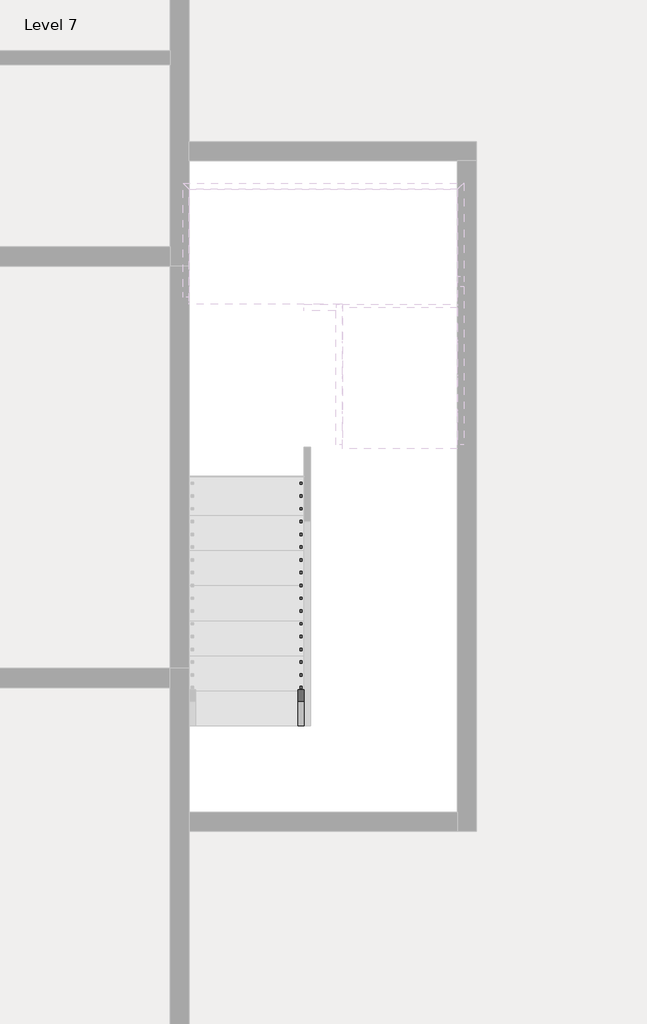
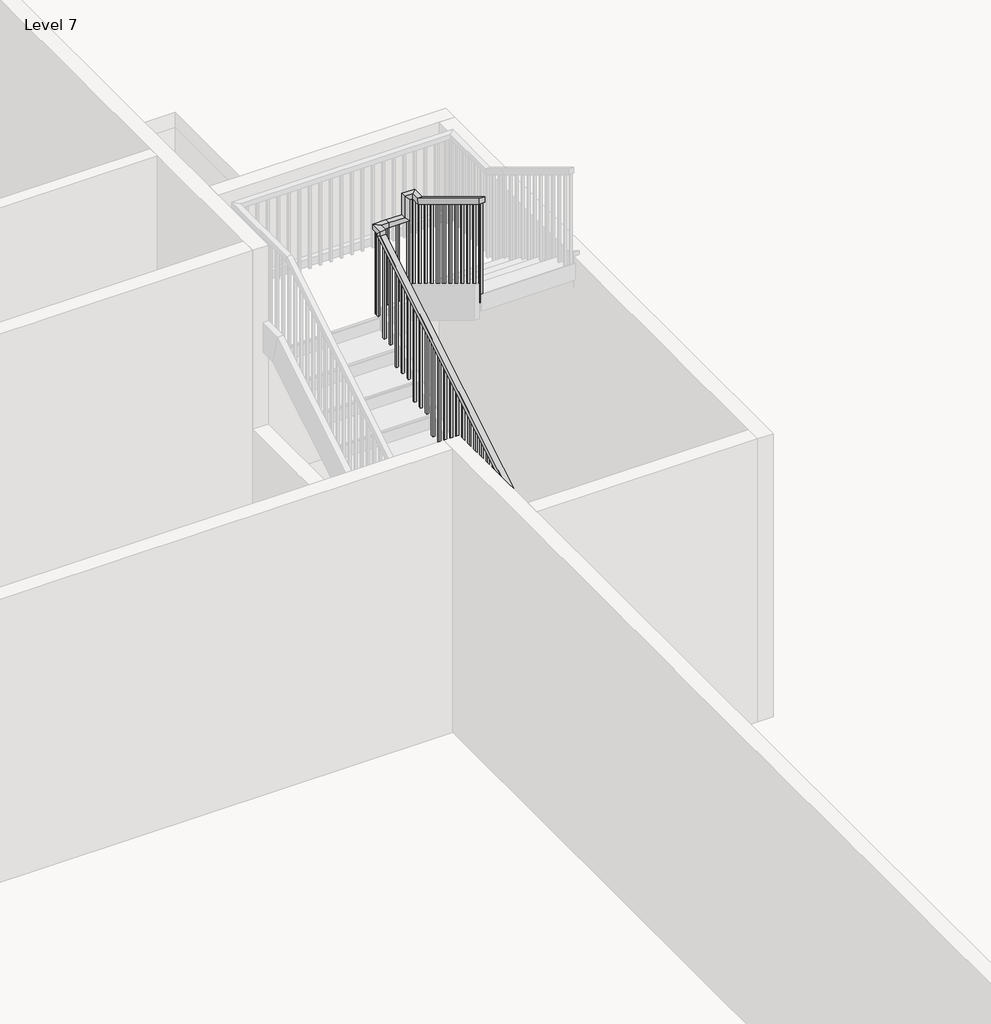
# One storey, part 7 of 8: 1 railing.
"""IFC4 building model written with IfcOpenShell, lengths in millimetres."""

from ifc_helpers import new_model, si_unit, frame, origin, place, context, project, spatial, polyline, outline, extrude, faceted_brep, element, save

model = new_model("IFC4")

# Units and contexts
model_context = context("Model", 3, world=origin())
ifc_project = project(units=[si_unit("LENGTHUNIT", "METRE", prefix="MILLI")], contexts=[model_context])

# Site, building, storey
site = spatial("IfcSite", under=ifc_project)
building = spatial("IfcBuilding", under=site)
storey = spatial("IfcBuildingStorey", under=building, Name="Level 7", Elevation=43522.6172466)

# Railing
placement = place(None, origin())
element("IfcRailing", 1, ObjectType="Handrail - Rectangular", at=placement, inside=storey, context=model_context, shape_type="SolidModel", body=[
    faceted_brep([(-2753.8415084, 19841.9216096, 44606.3505799), (-2753.8415084, 19841.9216096, 44546.9491197), (-2703.0415084, 19841.9216096, 44546.9491197), (-2703.0415084, 19841.9216096, 44606.3505799), (-2753.8415084, 23118.5216096, 46592.1687618), (-2753.8415084, 23169.3216096, 46563.5551803), (-2703.0415084, 23169.3216096, 46563.5551803), (-2703.0415084, 23118.5216096, 46592.1687618), (-2753.8415084, 23118.5216096, 46638.3505799), (-2753.8415084, 23169.3216096, 46587.5505799), (-2703.0415084, 23169.3216096, 46587.5505799), (-2703.0415084, 23118.5216096, 46638.3505799), (-2753.8415084, 23245.5216096, 46638.3505799), (-2753.8415084, 23245.5216096, 46587.5505799), (-2703.0415084, 23194.7216096, 46587.5505799), (-2703.0415084, 23194.7216096, 46638.3505799), (-2626.8415084, 23245.5216096, 46638.3505799), (-2626.8415084, 23245.5216096, 46587.5505799), (-2626.8415084, 23194.7216096, 46587.5505799), (-2626.8415084, 23194.7216096, 46638.3505799), (-2474.4415084, 23245.5216096, 46638.3505799), (-2423.6415084, 23245.5216096, 46587.5505799), (-2423.6415084, 23194.7216096, 46587.5505799), (-2474.4415084, 23194.7216096, 46638.3505799), (-2474.4415084, 23245.5216096, 46853.8657314), (-2423.6415084, 23245.5216096, 46803.0657314), (-2423.6415084, 23194.7216096, 46803.0657314), (-2474.4415084, 23194.7216096, 46853.8657314), (-2347.4415084, 23245.5216096, 46853.8657314), (-2347.4415084, 23245.5216096, 46803.0657314), (-2398.2415084, 23194.7216096, 46803.0657314), (-2398.2415084, 23194.7216096, 46853.8657314), (-2347.4415084, 23118.5216096, 46853.8657314), (-2347.4415084, 23104.3292002, 46803.0657314), (-2398.2415084, 23104.3292002, 46803.0657314), (-2398.2415084, 23118.5216096, 46853.8657314), (-2347.4415084, 22077.1216096, 47485.0172466), (-2398.2415084, 22077.1216096, 47485.0172466), (-2398.2415084, 22077.1216096, 47425.6157863), (-2347.4415084, 22077.1216096, 47425.6157863)], [[[0, 1, 2, 3]], [[1, 0, 4, 5]], [[2, 1, 5, 6]], [[3, 2, 6, 7]], [[0, 3, 7, 4]], [[5, 4, 8, 9]], [[6, 5, 9, 10]], [[7, 6, 10, 11]], [[4, 7, 11, 8]], [[9, 8, 12, 13]], [[10, 9, 13, 14]], [[11, 10, 14, 15]], [[8, 11, 15, 12]], [[13, 12, 16, 17]], [[14, 13, 17, 18]], [[15, 14, 18, 19]], [[12, 15, 19, 16]], [[17, 16, 20, 21]], [[18, 17, 21, 22]], [[19, 18, 22, 23]], [[16, 19, 23, 20]], [[21, 20, 24, 25]], [[22, 21, 25, 26]], [[23, 22, 26, 27]], [[20, 23, 27, 24]], [[25, 24, 28, 29]], [[26, 25, 29, 30]], [[27, 26, 30, 31]], [[24, 27, 31, 28]], [[29, 28, 32, 33]], [[30, 29, 33, 34]], [[31, 30, 34, 35]], [[28, 31, 35, 32]], [[36, 37, 38, 39]], [[33, 32, 36, 39]], [[34, 33, 39, 38]], [[35, 34, 38, 37]], [[32, 35, 37, 36]]]),
    extrude(outline(polyline([(22092.9966096, 47415.9945742), (22112.0466096, 47404.4491197), (22112.0466096, 46401.2839133), (22092.9966096, 46401.2839133), (22092.9966096, 47415.9945742)])), frame((-2382.3665084, 0.0, 0.0), z_axis=(1.0, 0.0, 0.0), x_axis=(0.0, 1.0, 0.0)), (0.0, 0.0, 1.0), 19.05),
    extrude(outline(polyline([(22194.5966096, 47354.4188166), (22213.6466096, 47342.8733621), (22213.6466096, 46401.2839133), (22194.5966096, 46401.2839133), (22194.5966096, 47354.4188166)])), frame((-2382.3665084, 0.0, 0.0), z_axis=(1.0, 0.0, 0.0), x_axis=(0.0, 1.0, 0.0)), (0.0, 0.0, 1.0), 19.05),
    extrude(outline(polyline([(22296.1966096, 47292.8430591), (22315.2466096, 47281.2976045), (22315.2466096, 46401.2839133), (22296.1966096, 46401.2839133), (22296.1966096, 47292.8430591)])), frame((-2382.3665084, 0.0, 0.0), z_axis=(1.0, 0.0, 0.0), x_axis=(0.0, 1.0, 0.0)), (0.0, 0.0, 1.0), 19.05),
    extrude(outline(polyline([(22397.7966096, 47231.2673015), (22416.8466096, 47219.721847), (22416.8466096, 46231.9505799), (22397.7966096, 46231.9505799), (22397.7966096, 47231.2673015)])), frame((-2382.3665084, 0.0, 0.0), z_axis=(1.0, 0.0, 0.0), x_axis=(0.0, 1.0, 0.0)), (0.0, 0.0, 1.0), 19.05),
    extrude(outline(polyline([(22499.3966096, 47169.6915439), (22518.4466096, 47158.1460894), (22518.4466096, 46231.9505799), (22499.3966096, 46231.9505799), (22499.3966096, 47169.6915439)])), frame((-2382.3665084, 0.0, 0.0), z_axis=(1.0, 0.0, 0.0), x_axis=(0.0, 1.0, 0.0)), (0.0, 0.0, 1.0), 19.05),
    extrude(outline(polyline([(22600.9966096, 47108.1157863), (22620.0466096, 47096.5703318), (22620.0466096, 46231.9505799), (22600.9966096, 46231.9505799), (22600.9966096, 47108.1157863)])), frame((-2382.3665084, 0.0, 0.0), z_axis=(1.0, 0.0, 0.0), x_axis=(0.0, 1.0, 0.0)), (0.0, 0.0, 1.0), 19.05),
    extrude(outline(polyline([(22702.5966096, 47046.5400288), (22721.6466096, 47034.9945742), (22721.6466096, 46062.6172466), (22702.5966096, 46062.6172466), (22702.5966096, 47046.5400288)])), frame((-2382.3665084, 0.0, 0.0), z_axis=(1.0, 0.0, 0.0), x_axis=(0.0, 1.0, 0.0)), (0.0, 0.0, 1.0), 19.05),
    extrude(outline(polyline([(22804.1966096, 46984.9642712), (22823.2466096, 46973.4188166), (22823.2466096, 46062.6172466), (22804.1966096, 46062.6172466), (22804.1966096, 46984.9642712)])), frame((-2382.3665084, 0.0, 0.0), z_axis=(1.0, 0.0, 0.0), x_axis=(0.0, 1.0, 0.0)), (0.0, 0.0, 1.0), 19.05),
    extrude(outline(polyline([(22905.7966096, 46923.3885136), (22924.8466096, 46911.8430591), (22924.8466096, 46062.6172466), (22905.7966096, 46062.6172466), (22905.7966096, 46923.3885136)])), frame((-2382.3665084, 0.0, 0.0), z_axis=(1.0, 0.0, 0.0), x_axis=(0.0, 1.0, 0.0)), (0.0, 0.0, 1.0), 19.05),
    extrude(outline(polyline([(23007.3966096, 46861.812756), (23026.4466096, 46850.2673015), (23026.4466096, 45893.2839133), (23007.3966096, 45893.2839133), (23007.3966096, 46861.812756)])), frame((-2382.3665084, 0.0, 0.0), z_axis=(1.0, 0.0, 0.0), x_axis=(0.0, 1.0, 0.0)), (0.0, 0.0, 1.0), 19.05),
    extrude(outline(polyline([(23108.9966096, 46800.2369985), (23128.0466096, 46788.6915439), (23128.0466096, 45893.2839133), (23108.9966096, 45893.2839133), (23108.9966096, 46800.2369985)])), frame((-2382.3665084, 0.0, 0.0), z_axis=(1.0, 0.0, 0.0), x_axis=(0.0, 1.0, 0.0)), (0.0, 0.0, 1.0), 19.05),
    extrude(outline(polyline([(-2433.1665084, 23210.5966096), (-2433.1665084, 23229.6466096), (-2414.1165084, 23229.6466096), (-2414.1165084, 23210.5966096), (-2433.1665084, 23210.5966096)])), frame((0.0, 0.0, 45723.9505799), z_axis=(0.0, 0.0, 1.0), x_axis=(1.0, 0.0, 0.0)), (0.0, 0.0, 1.0), 1079.1151515),
    extrude(outline(polyline([(-2534.7665084, 23210.5966096), (-2534.7665084, 23229.6466096), (-2515.7165084, 23229.6466096), (-2515.7165084, 23210.5966096), (-2534.7665084, 23210.5966096)])), frame((0.0, 0.0, 45723.9505799), z_axis=(0.0, 0.0, 1.0), x_axis=(1.0, 0.0, 0.0)), (0.0, 0.0, 1.0), 863.6),
    extrude(outline(polyline([(-2636.3665084, 23210.5966096), (-2636.3665084, 23229.6466096), (-2617.3165084, 23229.6466096), (-2617.3165084, 23210.5966096), (-2636.3665084, 23210.5966096)])), frame((0.0, 0.0, 45723.9505799), z_axis=(0.0, 0.0, 1.0), x_axis=(1.0, 0.0, 0.0)), (0.0, 0.0, 1.0), 863.6),
    extrude(outline(polyline([(-2718.9165084, 23185.1966096), (-2737.9665084, 23185.1966096), (-2737.9665084, 23204.2466096), (-2718.9165084, 23204.2466096), (-2718.9165084, 23185.1966096)])), frame((0.0, 0.0, 45723.9505799), z_axis=(0.0, 0.0, 1.0), x_axis=(1.0, 0.0, 0.0)), (0.0, 0.0, 1.0), 863.6),
    extrude(outline(polyline([(23083.5966096, 46511.6006348), (23102.6466096, 46523.1460894), (23102.6466096, 45554.6172466), (23083.5966096, 45554.6172466), (23083.5966096, 46511.6006348)])), frame((-2737.9665084, 0.0, 0.0), z_axis=(1.0, 0.0, 0.0), x_axis=(0.0, 1.0, 0.0)), (0.0, 0.0, 1.0), 19.05),
    extrude(outline(polyline([(22981.9966096, 46450.0248773), (23001.0466096, 46461.5703318), (23001.0466096, 45554.6172466), (22981.9966096, 45554.6172466), (22981.9966096, 46450.0248773)])), frame((-2737.9665084, 0.0, 0.0), z_axis=(1.0, 0.0, 0.0), x_axis=(0.0, 1.0, 0.0)), (0.0, 0.0, 1.0), 19.05),
    extrude(outline(polyline([(22880.3966096, 46388.4491197), (22899.4466096, 46399.9945742), (22899.4466096, 45385.2839133), (22880.3966096, 45385.2839133), (22880.3966096, 46388.4491197)])), frame((-2737.9665084, 0.0, 0.0), z_axis=(1.0, 0.0, 0.0), x_axis=(0.0, 1.0, 0.0)), (0.0, 0.0, 1.0), 19.05),
    extrude(outline(polyline([(22778.7966096, 46326.8733621), (22797.8466096, 46338.4188166), (22797.8466096, 45385.2839133), (22778.7966096, 45385.2839133), (22778.7966096, 46326.8733621)])), frame((-2737.9665084, 0.0, 0.0), z_axis=(1.0, 0.0, 0.0), x_axis=(0.0, 1.0, 0.0)), (0.0, 0.0, 1.0), 19.05),
    extrude(outline(polyline([(22677.1966096, 46265.2976045), (22696.2466096, 46276.8430591), (22696.2466096, 45385.2839133), (22677.1966096, 45385.2839133), (22677.1966096, 46265.2976045)])), frame((-2737.9665084, 0.0, 0.0), z_axis=(1.0, 0.0, 0.0), x_axis=(0.0, 1.0, 0.0)), (0.0, 0.0, 1.0), 19.05),
    extrude(outline(polyline([(22575.5966096, 46203.721847), (22594.6466096, 46215.2673015), (22594.6466096, 45215.9505799), (22575.5966096, 45215.9505799), (22575.5966096, 46203.721847)])), frame((-2737.9665084, 0.0, 0.0), z_axis=(1.0, 0.0, 0.0), x_axis=(0.0, 1.0, 0.0)), (0.0, 0.0, 1.0), 19.05),
    extrude(outline(polyline([(22473.9966096, 46142.1460894), (22493.0466096, 46153.6915439), (22493.0466096, 45215.9505799), (22473.9966096, 45215.9505799), (22473.9966096, 46142.1460894)])), frame((-2737.9665084, 0.0, 0.0), z_axis=(1.0, 0.0, 0.0), x_axis=(0.0, 1.0, 0.0)), (0.0, 0.0, 1.0), 19.05),
    extrude(outline(polyline([(22372.3966096, 46080.5703318), (22391.4466096, 46092.1157863), (22391.4466096, 45215.9505799), (22372.3966096, 45215.9505799), (22372.3966096, 46080.5703318)])), frame((-2737.9665084, 0.0, 0.0), z_axis=(1.0, 0.0, 0.0), x_axis=(0.0, 1.0, 0.0)), (0.0, 0.0, 1.0), 19.05),
    extrude(outline(polyline([(22270.7966096, 46018.9945742), (22289.8466096, 46030.5400288), (22289.8466096, 45046.6172466), (22270.7966096, 45046.6172466), (22270.7966096, 46018.9945742)])), frame((-2737.9665084, 0.0, 0.0), z_axis=(1.0, 0.0, 0.0), x_axis=(0.0, 1.0, 0.0)), (0.0, 0.0, 1.0), 19.05),
    extrude(outline(polyline([(22169.1966096, 45957.4188166), (22188.2466096, 45968.9642712), (22188.2466096, 45046.6172466), (22169.1966096, 45046.6172466), (22169.1966096, 45957.4188166)])), frame((-2737.9665084, 0.0, 0.0), z_axis=(1.0, 0.0, 0.0), x_axis=(0.0, 1.0, 0.0)), (0.0, 0.0, 1.0), 19.05),
    extrude(outline(polyline([(22067.5966096, 45895.8430591), (22086.6466096, 45907.3885136), (22086.6466096, 45046.6172466), (22067.5966096, 45046.6172466), (22067.5966096, 45895.8430591)])), frame((-2737.9665084, 0.0, 0.0), z_axis=(1.0, 0.0, 0.0), x_axis=(0.0, 1.0, 0.0)), (0.0, 0.0, 1.0), 19.05),
    extrude(outline(polyline([(21965.9966096, 45834.2673015), (21985.0466096, 45845.812756), (21985.0466096, 44877.2839133), (21965.9966096, 44877.2839133), (21965.9966096, 45834.2673015)])), frame((-2737.9665084, 0.0, 0.0), z_axis=(1.0, 0.0, 0.0), x_axis=(0.0, 1.0, 0.0)), (0.0, 0.0, 1.0), 19.05),
    extrude(outline(polyline([(21864.3966096, 45772.6915439), (21883.4466096, 45784.2369985), (21883.4466096, 44877.2839133), (21864.3966096, 44877.2839133), (21864.3966096, 45772.6915439)])), frame((-2737.9665084, 0.0, 0.0), z_axis=(1.0, 0.0, 0.0), x_axis=(0.0, 1.0, 0.0)), (0.0, 0.0, 1.0), 19.05),
    extrude(outline(polyline([(21762.7966096, 45711.1157863), (21781.8466096, 45722.6612409), (21781.8466096, 44707.9505799), (21762.7966096, 44707.9505799), (21762.7966096, 45711.1157863)])), frame((-2737.9665084, 0.0, 0.0), z_axis=(1.0, 0.0, 0.0), x_axis=(0.0, 1.0, 0.0)), (0.0, 0.0, 1.0), 19.05),
    extrude(outline(polyline([(21661.1966096, 45649.5400288), (21680.2466096, 45661.0854833), (21680.2466096, 44707.9505799), (21661.1966096, 44707.9505799), (21661.1966096, 45649.5400288)])), frame((-2737.9665084, 0.0, 0.0), z_axis=(1.0, 0.0, 0.0), x_axis=(0.0, 1.0, 0.0)), (0.0, 0.0, 1.0), 19.05),
    extrude(outline(polyline([(21559.5966096, 45587.9642712), (21578.6466096, 45599.5097257), (21578.6466096, 44707.9505799), (21559.5966096, 44707.9505799), (21559.5966096, 45587.9642712)])), frame((-2737.9665084, 0.0, 0.0), z_axis=(1.0, 0.0, 0.0), x_axis=(0.0, 1.0, 0.0)), (0.0, 0.0, 1.0), 19.05),
    extrude(outline(polyline([(21457.9966096, 45526.3885136), (21477.0466096, 45537.9339682), (21477.0466096, 44538.6172466), (21457.9966096, 44538.6172466), (21457.9966096, 45526.3885136)])), frame((-2737.9665084, 0.0, 0.0), z_axis=(1.0, 0.0, 0.0), x_axis=(0.0, 1.0, 0.0)), (0.0, 0.0, 1.0), 19.05),
    extrude(outline(polyline([(21356.3966096, 45464.812756), (21375.4466096, 45476.3582106), (21375.4466096, 44538.6172466), (21356.3966096, 44538.6172466), (21356.3966096, 45464.812756)])), frame((-2737.9665084, 0.0, 0.0), z_axis=(1.0, 0.0, 0.0), x_axis=(0.0, 1.0, 0.0)), (0.0, 0.0, 1.0), 19.05),
    extrude(outline(polyline([(21254.7966096, 45403.2369985), (21273.8466096, 45414.782453), (21273.8466096, 44538.6172466), (21254.7966096, 44538.6172466), (21254.7966096, 45403.2369985)])), frame((-2737.9665084, 0.0, 0.0), z_axis=(1.0, 0.0, 0.0), x_axis=(0.0, 1.0, 0.0)), (0.0, 0.0, 1.0), 19.05),
    extrude(outline(polyline([(21153.1966096, 45341.6612409), (21172.2466096, 45353.2066954), (21172.2466096, 44369.2839133), (21153.1966096, 44369.2839133), (21153.1966096, 45341.6612409)])), frame((-2737.9665084, 0.0, 0.0), z_axis=(1.0, 0.0, 0.0), x_axis=(0.0, 1.0, 0.0)), (0.0, 0.0, 1.0), 19.05),
    extrude(outline(polyline([(21051.5966096, 45280.0854833), (21070.6466096, 45291.6309379), (21070.6466096, 44369.2839133), (21051.5966096, 44369.2839133), (21051.5966096, 45280.0854833)])), frame((-2737.9665084, 0.0, 0.0), z_axis=(1.0, 0.0, 0.0), x_axis=(0.0, 1.0, 0.0)), (0.0, 0.0, 1.0), 19.05),
    extrude(outline(polyline([(20949.9966096, 45218.5097257), (20969.0466096, 45230.0551803), (20969.0466096, 44369.2839133), (20949.9966096, 44369.2839133), (20949.9966096, 45218.5097257)])), frame((-2737.9665084, 0.0, 0.0), z_axis=(1.0, 0.0, 0.0), x_axis=(0.0, 1.0, 0.0)), (0.0, 0.0, 1.0), 19.05),
    extrude(outline(polyline([(20848.3966096, 45156.9339682), (20867.4466096, 45168.4794227), (20867.4466096, 44199.9505799), (20848.3966096, 44199.9505799), (20848.3966096, 45156.9339682)])), frame((-2737.9665084, 0.0, 0.0), z_axis=(1.0, 0.0, 0.0), x_axis=(0.0, 1.0, 0.0)), (0.0, 0.0, 1.0), 19.05),
    extrude(outline(polyline([(20746.7966096, 45095.3582106), (20765.8466096, 45106.9036651), (20765.8466096, 44199.9505799), (20746.7966096, 44199.9505799), (20746.7966096, 45095.3582106)])), frame((-2737.9665084, 0.0, 0.0), z_axis=(1.0, 0.0, 0.0), x_axis=(0.0, 1.0, 0.0)), (0.0, 0.0, 1.0), 19.05),
    extrude(outline(polyline([(20645.1966096, 45033.782453), (20664.2466096, 45045.3279076), (20664.2466096, 44030.6172466), (20645.1966096, 44030.6172466), (20645.1966096, 45033.782453)])), frame((-2737.9665084, 0.0, 0.0), z_axis=(1.0, 0.0, 0.0), x_axis=(0.0, 1.0, 0.0)), (0.0, 0.0, 1.0), 19.05),
    extrude(outline(polyline([(20543.5966096, 44972.2066954), (20562.6466096, 44983.75215), (20562.6466096, 44030.6172466), (20543.5966096, 44030.6172466), (20543.5966096, 44972.2066954)])), frame((-2737.9665084, 0.0, 0.0), z_axis=(1.0, 0.0, 0.0), x_axis=(0.0, 1.0, 0.0)), (0.0, 0.0, 1.0), 19.05),
    extrude(outline(polyline([(20441.9966096, 44910.6309379), (20461.0466096, 44922.1763924), (20461.0466096, 44030.6172466), (20441.9966096, 44030.6172466), (20441.9966096, 44910.6309379)])), frame((-2737.9665084, 0.0, 0.0), z_axis=(1.0, 0.0, 0.0), x_axis=(0.0, 1.0, 0.0)), (0.0, 0.0, 1.0), 19.05),
    extrude(outline(polyline([(20340.3966096, 44849.0551803), (20359.4466096, 44860.6006348), (20359.4466096, 43861.2839133), (20340.3966096, 43861.2839133), (20340.3966096, 44849.0551803)])), frame((-2737.9665084, 0.0, 0.0), z_axis=(1.0, 0.0, 0.0), x_axis=(0.0, 1.0, 0.0)), (0.0, 0.0, 1.0), 19.05),
    extrude(outline(polyline([(20238.7966096, 44787.4794227), (20257.8466096, 44799.0248773), (20257.8466096, 43861.2839133), (20238.7966096, 43861.2839133), (20238.7966096, 44787.4794227)])), frame((-2737.9665084, 0.0, 0.0), z_axis=(1.0, 0.0, 0.0), x_axis=(0.0, 1.0, 0.0)), (0.0, 0.0, 1.0), 19.05),
    extrude(outline(polyline([(20137.1966096, 44725.9036651), (20156.2466096, 44737.4491197), (20156.2466096, 43861.2839133), (20137.1966096, 43861.2839133), (20137.1966096, 44725.9036651)])), frame((-2737.9665084, 0.0, 0.0), z_axis=(1.0, 0.0, 0.0), x_axis=(0.0, 1.0, 0.0)), (0.0, 0.0, 1.0), 19.05),
    extrude(outline(polyline([(20035.5966096, 44664.3279076), (20054.6466096, 44675.8733621), (20054.6466096, 43691.9505799), (20035.5966096, 43691.9505799), (20035.5966096, 44664.3279076)])), frame((-2737.9665084, 0.0, 0.0), z_axis=(1.0, 0.0, 0.0), x_axis=(0.0, 1.0, 0.0)), (0.0, 0.0, 1.0), 19.05),
    extrude(outline(polyline([(19933.9966096, 44602.75215), (19953.0466096, 44614.2976045), (19953.0466096, 43691.9505799), (19933.9966096, 43691.9505799), (19933.9966096, 44602.75215)])), frame((-2737.9665084, 0.0, 0.0), z_axis=(1.0, 0.0, 0.0), x_axis=(0.0, 1.0, 0.0)), (0.0, 0.0, 1.0), 19.05),
    extrude(outline(polyline([(-2382.3665084, 23210.5966096), (-2382.3665084, 23229.6466096), (-2363.3165084, 23229.6466096), (-2363.3165084, 23210.5966096), (-2382.3665084, 23210.5966096)])), frame((0.0, 0.0, 45723.9505799), z_axis=(0.0, 0.0, 1.0), x_axis=(1.0, 0.0, 0.0)), (0.0, 0.0, 1.0), 1079.1151515),
    extrude(outline(polyline([(-2718.9165084, 23210.5966096), (-2737.9665084, 23210.5966096), (-2737.9665084, 23229.6466096), (-2718.9165084, 23229.6466096), (-2718.9165084, 23210.5966096)])), frame((0.0, 0.0, 45723.9505799), z_axis=(0.0, 0.0, 1.0), x_axis=(1.0, 0.0, 0.0)), (0.0, 0.0, 1.0), 863.6),
    extrude(outline(polyline([(22077.1216096, 47425.6157863), (22096.1716096, 47414.0703318), (22096.1716096, 46401.2839133), (22077.1216096, 46401.2839133), (22077.1216096, 47425.6157863)])), frame((-2382.3665084, 0.0, 0.0), z_axis=(1.0, 0.0, 0.0), x_axis=(0.0, 1.0, 0.0)), (0.0, 0.0, 1.0), 19.05),
    extrude(outline(polyline([(19841.9216096, 44546.9491197), (19860.9716096, 44558.4945742), (19860.9716096, 43691.9505799), (19841.9216096, 43691.9505799), (19841.9216096, 44546.9491197)])), frame((-2737.9665084, 0.0, 0.0), z_axis=(1.0, 0.0, 0.0), x_axis=(0.0, 1.0, 0.0)), (0.0, 0.0, 1.0), 19.05),
])

save(model, "model.ifc")

# Revit data of these elements
# Type "Handrail - Rectangular"
#   Assembly Code = "C2010400"
#   built-in parameter 1008612 = 0.0416667 (stored number, unit not read)
#   built-in parameter 1008611 = 0.0416667 (stored number, unit not read)
#   built-in parameter 1008609 = 0.333333 (stored number, unit not read)
#   built-in parameter 1008604 = 0.166667 (stored number, unit not read)
#   built-in parameter 1008603 = 0.166667 (stored number, unit not read)
#   Railing Height = 3' - 0"
#   built-in parameter 1008630 = 2
#   built-in parameter 1008610 = 2
#   built-in parameter 1008618 = Baluster - Square : 3/4"
# Element 1 (IfcRailing, "Handrail - Rectangular")
#   Phase Created = New Construction
